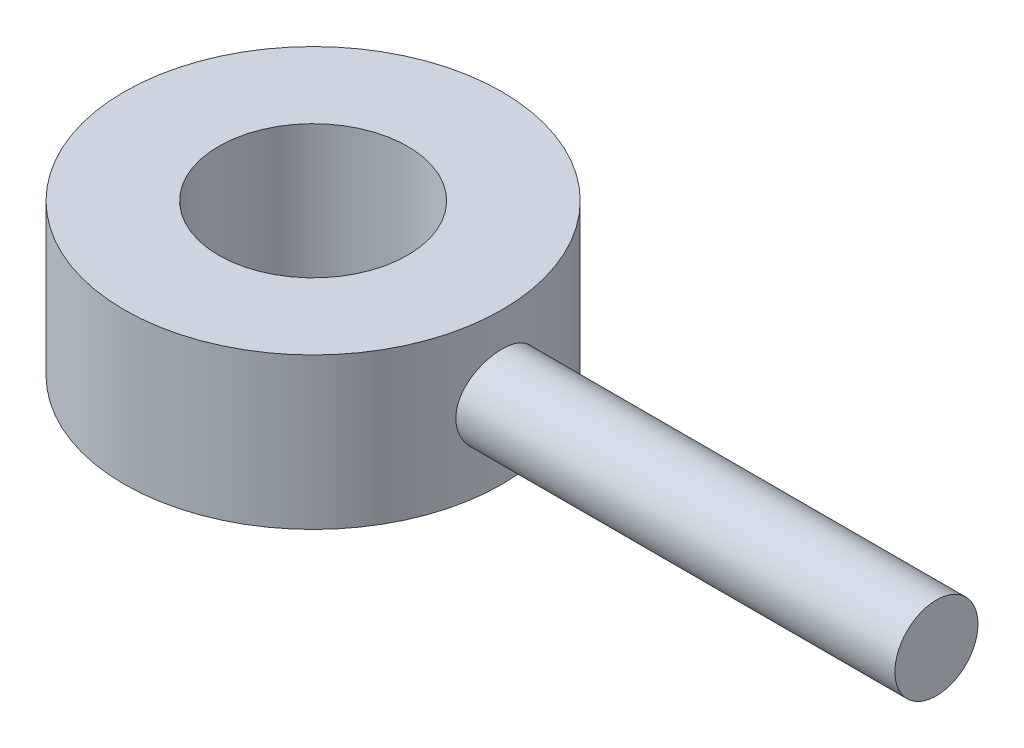
SolidWorks part; units mm, degrees
material "Plain Carbon Steel"
ref_plane "Front Plane" through (0, 0, 0) normal (0, 0, 1) x (1, 0, 0)
ref_plane "Top Plane" through (0, 0, 0) normal (0, 1, 0) x (1, 0, 0)
ref_plane "Right Plane" through (0, 0, 0) normal (1, 0, 0) x (0, 0, -1)
sketch "Hub Ring Sketch" plane through (0, 0, 0) normal (0, 1, 0) x (1, 0, 0)
  circle A0 centre (0, 0) radius 5
  circle A1 centre (0, 0) radius 2.5
  dimension "D1" = 10
  dimension "D2" = 5
extrude "Hub Ring Ø10xØ5" add sketch "Hub Ring Sketch" along normal blind 4
ref_plane "Arm Start Plane" through (5, 0, 0) normal (1, 0, 0) x (0, 0, -1)
sketch "Arm Rod Sketch" plane through (5, 0, 0) normal (1, 0, 0) x (0, 0, -1)
  circle A0 centre (0, 2) radius 1.1
  dimension "D1" = 2.2
  dimension "D2" = 2
extrude "Arm Rod Ø2.2" add sketch "Arm Rod Sketch" along normal blind 11.5 separate body
sketch "Arm Root Sketch" plane through (5, 0, 0) normal (1, 0, 0) x (0, 0, -1)
  circle A0 centre (0, 2) radius 1.1 construction
  circle A1 centre (0, 2) radius 1.1
extrude "Arm Root Joint" add sketch "Arm Root Sketch" against normal blind 2.5
